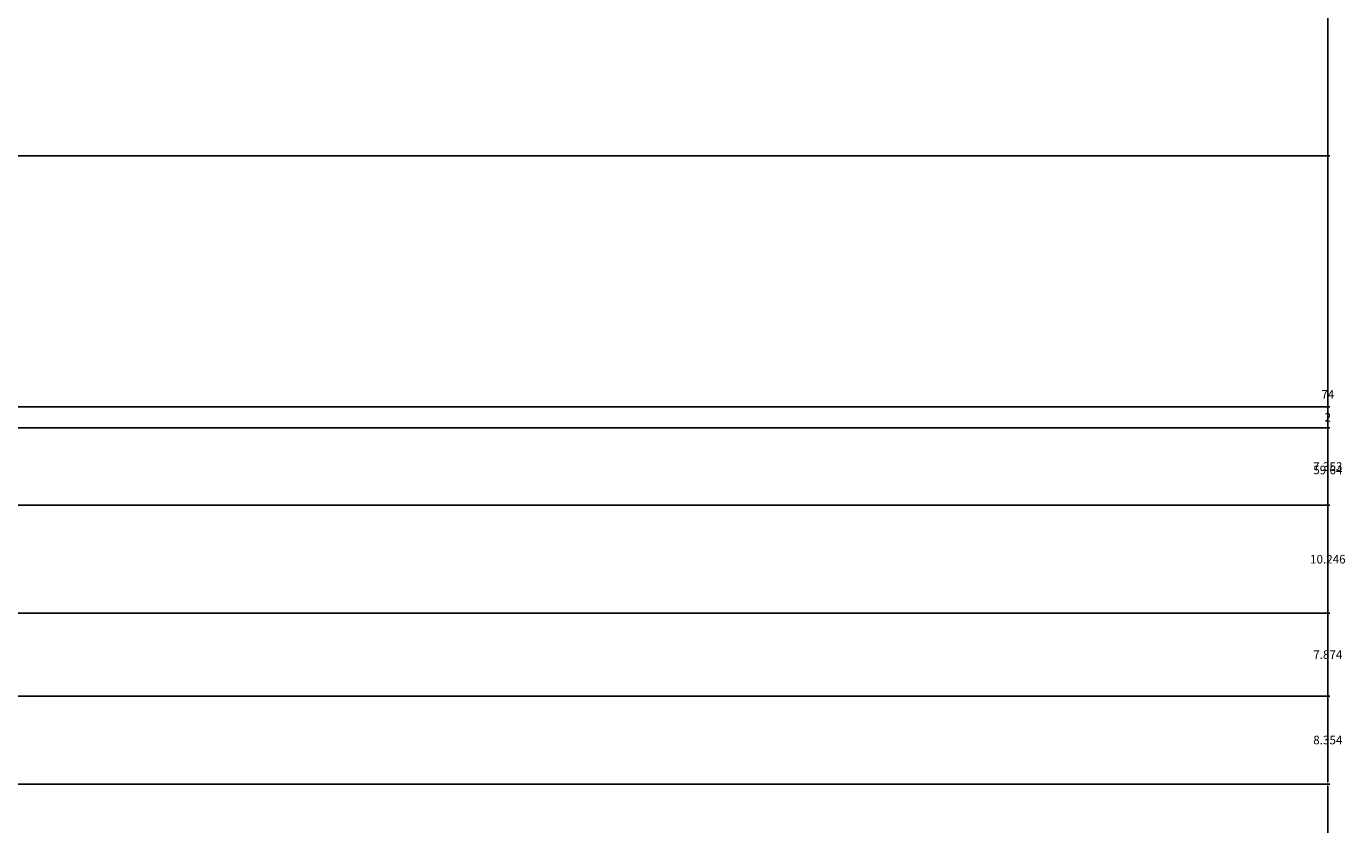
# Model space of a CAD drawing. Units: inches. Extents: x 36 to 594, y 79 to 831.
# Tile 29 of 30: x 469 to 594, y 590 to 666. Entities that reach past the tile are written whole.
import ezdxf

# ---------------------------------------------------------------- set-up
doc = ezdxf.new("R2010")
doc.units = ezdxf.units.IN
doc.header["$MEASUREMENT"] = 0
doc.layers.add('A-ANNO-DIMS', color=2, linetype='Continuous', lineweight=18)
doc.styles.get("Standard").update_dxf_attribs({"font": 'arial.ttf'})
doc.dimstyles.get("Standard").update_dxf_attribs({"dimtxt": 0.8125, "dimasz": 0.18, "dimexe": 0.18, "dimexo": 0.0625, "dimgap": 0.09, "dimtad": 0, "dimtih": 1, "dimtoh": 1, "dimdec": 4, "dimzin": 0, "dimdsep": 46, "dimlunit": 4, "dimtxsty": 'Standard', "dimcen": 0.09, "dimadec": 0, "dimazin": 0, "dimtfac": 1, "dimtdec": 4, "dimtofl": 0, "dimtmove": 0, "dimatfit": 3, "dimfxl": 1, "dimtolj": 1, "dimtzin": 0, "dimarcsym": 0})

# ---------------------------------------------------------------- blocks, each defined once
blk = doc.blocks.new('*D35')
at = {"layer": 'A-ANNO-DIMS', "color": 0, "lineweight": -2, "transparency": 16777216}
for p, q in [((424.56, 594.21), (592.85, 594.21)), ((592.67, 594.03), (592.67, 522.71)), ((592.67, 450.39), (592.67, 521.71)), ((448.45, 450.21), (592.85, 450.21))]:
    blk.add_line(p, q, dxfattribs=at)
at = {"layer": 'A-ANNO-DIMS', "color": 0, "transparency": 16777216}
for points in [[(592.64, 594.03), (592.7, 594.03), (592.67, 594.21)], [(592.64, 450.39), (592.7, 450.39), (592.67, 450.21)]]:
    blk.add_solid(points, dxfattribs=at)
at = {"layer": 'Defpoints', "color": 0, "transparency": 16777216}
for p in [(424.5, 594.21), (592.67, 594.21), (448.39, 450.21)]:
    blk.add_point(p, dxfattribs=at)
at = {"layer": 'A-ANNO-DIMS', "color": 0, "transparency": 16777216, "insert": (592.67, 522.21), "char_height": 0.812, "attachment_point": 5}
blk.add_mtext('\\A1;144', dxfattribs=at)
blk = doc.blocks.new('*D36')
at = {"layer": 'A-ANNO-DIMS', "color": 0, "lineweight": -2, "transparency": 16777216}
for p, q in [((448.452274, 668.212359), (592.848908, 668.212359)), ((592.668908, 668.032359), (592.668908, 631.708609)), ((592.668908, 594.392359), (592.668908, 630.716109)), ((424.55834, 594.212359), (592.848908, 594.212359))]:
    blk.add_line(p, q, dxfattribs=at)
at = {"layer": 'A-ANNO-DIMS', "color": 0, "transparency": 16777216}
for points in [[(592.638908, 668.032359), (592.698908, 668.032359), (592.668908, 668.212359)], [(592.638908, 594.392359), (592.698908, 594.392359), (592.668908, 594.212359)]]:
    blk.add_solid(points, dxfattribs=at)
at = {"layer": 'Defpoints', "color": 0, "transparency": 16777216}
for p in [(448.389774, 668.212359), (592.668908, 668.212359), (424.49584, 594.212359)]:
    blk.add_point(p, dxfattribs=at)
at = {"layer": 'A-ANNO-DIMS', "color": 0, "transparency": 16777216, "insert": (592.668908, 631.212359), "char_height": 0.8125, "attachment_point": 5}
blk.add_mtext('\\A1;74', dxfattribs=at)
blk = doc.blocks.new('*D40')
at = {"layer": 'A-ANNO-DIMS', "color": 0, "lineweight": -2, "transparency": 16777216}
for p, q in [((413.27, 653.86), (592.85, 653.86)), ((592.67, 653.68), (592.67, 624.54)), ((592.67, 594.39), (592.67, 623.53)), ((424.56, 594.21), (592.85, 594.21))]:
    blk.add_line(p, q, dxfattribs=at)
at = {"layer": 'A-ANNO-DIMS', "color": 0, "transparency": 16777216}
for points in [[(592.64, 653.68), (592.7, 653.68), (592.67, 653.86)], [(592.64, 594.39), (592.7, 594.39), (592.67, 594.21)]]:
    blk.add_solid(points, dxfattribs=at)
at = {"layer": 'Defpoints', "color": 0, "transparency": 16777216}
for p in [(413.2, 653.86), (592.67, 653.86), (424.5, 594.21)]:
    blk.add_point(p, dxfattribs=at)
at = {"layer": 'A-ANNO-DIMS', "color": 0, "transparency": 16777216, "insert": (592.67, 624.03), "char_height": 0.812, "attachment_point": 5}
blk.add_mtext('\\A1;59.64', dxfattribs=at)
blk = doc.blocks.new('*D117')
at = {"layer": 'A-ANNO-DIMS', "color": 0, "lineweight": -2, "transparency": 16777216}
for p, q in [((341.9, 602.57), (592.85, 602.57)), ((592.67, 602.39), (592.67, 598.89)), ((592.67, 594.39), (592.67, 597.88)), ((341.9, 594.21), (592.85, 594.21))]:
    blk.add_line(p, q, dxfattribs=at)
at = {"layer": 'A-ANNO-DIMS', "color": 0, "transparency": 16777216}
for points in [[(592.64, 602.39), (592.7, 602.39), (592.67, 602.57)], [(592.64, 594.39), (592.7, 594.39), (592.67, 594.21)]]:
    blk.add_solid(points, dxfattribs=at)
at = {"layer": 'Defpoints', "color": 0, "transparency": 16777216}
for p in [(341.84, 602.57), (592.67, 602.57), (341.84, 594.21)]:
    blk.add_point(p, dxfattribs=at)
at = {"layer": 'A-ANNO-DIMS', "color": 0, "transparency": 16777216, "insert": (592.67, 598.39), "char_height": 0.812, "attachment_point": 5}
blk.add_mtext('\\A1;8.354', dxfattribs=at)
blk = doc.blocks.new('*D118')
at = {"layer": 'A-ANNO-DIMS', "color": 0, "lineweight": -2, "transparency": 16777216}
for p, q in [((341.9, 610.44), (592.85, 610.44)), ((592.67, 610.26), (592.67, 607.01)), ((592.67, 602.75), (592.67, 606)), ((341.9, 602.57), (592.85, 602.57))]:
    blk.add_line(p, q, dxfattribs=at)
at = {"layer": 'A-ANNO-DIMS', "color": 0, "transparency": 16777216}
for points in [[(592.64, 610.26), (592.7, 610.26), (592.67, 610.44)], [(592.64, 602.75), (592.7, 602.75), (592.67, 602.57)]]:
    blk.add_solid(points, dxfattribs=at)
at = {"layer": 'Defpoints', "color": 0, "transparency": 16777216}
for p in [(341.84, 610.44), (592.67, 610.44), (341.84, 602.57)]:
    blk.add_point(p, dxfattribs=at)
at = {"layer": 'A-ANNO-DIMS', "color": 0, "transparency": 16777216, "insert": (592.67, 606.5), "char_height": 0.812, "attachment_point": 5}
blk.add_mtext('\\A1;7.874', dxfattribs=at)
blk = doc.blocks.new('*D119')
at = {"layer": 'A-ANNO-DIMS', "color": 0, "lineweight": -2, "transparency": 16777216}
for p, q in [((341.9, 620.69), (592.85, 620.69)), ((592.67, 620.51), (592.67, 616.07)), ((592.67, 610.62), (592.67, 615.06)), ((341.9, 610.44), (592.85, 610.44))]:
    blk.add_line(p, q, dxfattribs=at)
at = {"layer": 'A-ANNO-DIMS', "color": 0, "transparency": 16777216}
for points in [[(592.64, 620.51), (592.7, 620.51), (592.67, 620.69)], [(592.64, 610.62), (592.7, 610.62), (592.67, 610.44)]]:
    blk.add_solid(points, dxfattribs=at)
at = {"layer": 'Defpoints', "color": 0, "transparency": 16777216}
for p in [(341.84, 620.69), (592.67, 620.69), (341.84, 610.44)]:
    blk.add_point(p, dxfattribs=at)
at = {"layer": 'A-ANNO-DIMS', "color": 0, "transparency": 16777216, "insert": (592.67, 615.56), "char_height": 0.812, "attachment_point": 5}
blk.add_mtext('\\A1;10.246', dxfattribs=at)
blk = doc.blocks.new('*D120')
at = {"layer": 'A-ANNO-DIMS', "color": 0, "lineweight": -2, "transparency": 16777216}
for p, q in [((341.9, 628.04), (592.85, 628.04)), ((592.67, 627.86), (592.67, 624.87)), ((592.67, 620.87), (592.67, 623.86)), ((341.9, 620.69), (592.85, 620.69))]:
    blk.add_line(p, q, dxfattribs=at)
at = {"layer": 'A-ANNO-DIMS', "color": 0, "transparency": 16777216}
for points in [[(592.64, 627.86), (592.7, 627.86), (592.67, 628.04)], [(592.64, 620.87), (592.7, 620.87), (592.67, 620.69)]]:
    blk.add_solid(points, dxfattribs=at)
at = {"layer": 'Defpoints', "color": 0, "transparency": 16777216}
for p in [(341.84, 628.04), (592.67, 628.04), (341.84, 620.69)]:
    blk.add_point(p, dxfattribs=at)
at = {"layer": 'A-ANNO-DIMS', "color": 0, "transparency": 16777216, "insert": (592.67, 624.36), "char_height": 0.812, "attachment_point": 5}
blk.add_mtext('\\A1;7.353', dxfattribs=at)
blk = doc.blocks.new('*D121')
at = {"layer": 'A-ANNO-DIMS', "color": 0, "lineweight": -2, "transparency": 16777216}
for p, q in [((341.9, 630.04), (592.85, 630.04)), ((592.67, 629.86), (592.67, 629.54)), ((341.9, 628.04), (592.85, 628.04)), ((592.67, 628.22), (592.67, 628.54))]:
    blk.add_line(p, q, dxfattribs=at)
at = {"layer": 'A-ANNO-DIMS', "color": 0, "transparency": 16777216}
for points in [[(592.64, 629.86), (592.7, 629.86), (592.67, 630.04)], [(592.64, 628.22), (592.7, 628.22), (592.67, 628.04)]]:
    blk.add_solid(points, dxfattribs=at)
at = {"layer": 'Defpoints', "color": 0, "transparency": 16777216}
for p in [(341.84, 630.04), (592.67, 630.04), (341.84, 628.04)]:
    blk.add_point(p, dxfattribs=at)
at = {"layer": 'A-ANNO-DIMS', "color": 0, "transparency": 16777216, "insert": (592.67, 629.04), "char_height": 0.812, "attachment_point": 5}
blk.add_mtext('\\A1;2', dxfattribs=at)

msp = doc.modelspace()

# ---------------------------------------------------------------- dimensions: what is measured, and where the dimension line sits
at = {"layer": 'A-ANNO-DIMS'}
for base, p1, p2, override, picture, middle in [((592.6689, 668.2124), (424.4958, 594.2124), (448.3898, 668.2124), {"dimdec": 0, "dimlfac": 1, "dimrnd": 0, "dimzin": 0, "dimdsep": 46, "dimlunit": 2}, '*D36', (592.6689, 631.2124)), ((592.6689, 653.8563), (424.4958, 594.2124), (413.2033, 653.8563), {"dimdec": 2, "dimlfac": 1, "dimrnd": 0, "dimzin": 0, "dimdsep": 46, "dimlunit": 2}, '*D40', (592.6689, 624.0344)), ((592.6689, 630.0394), (341.8367, 628.0394), (341.8367, 630.0394), {"dimdec": 0, "dimlfac": 1, "dimrnd": 0, "dimzin": 0, "dimdsep": 46, "dimlunit": 2}, '*D121', (592.6689, 629.0394)), ((592.6689, 628.0394), (341.8367, 620.6866), (341.8367, 628.0394), {"dimdec": 3, "dimlfac": 1, "dimrnd": 0, "dimzin": 0, "dimdsep": 46, "dimlunit": 2}, '*D120', (592.6689, 624.363)), ((592.6689, 620.6866), (341.8367, 610.4402), (341.8367, 620.6866), {"dimdec": 3, "dimlfac": 1, "dimrnd": 0, "dimzin": 0, "dimdsep": 46, "dimlunit": 2}, '*D119', (592.6689, 615.5634)), ((592.66891, 610.44025), (341.83669, 602.56672), (341.83669, 610.44025), {"dimdec": 3, "dimlfac": 1, "dimrnd": 0, "dimzin": 0, "dimdsep": 46, "dimlunit": 2}, '*D118', (592.66891, 606.50348)), ((592.6689, 602.5667), (341.8367, 594.2124), (341.8367, 602.5667), {"dimdec": 3, "dimlfac": 1, "dimrnd": 0, "dimzin": 0, "dimdsep": 46, "dimlunit": 2}, '*D117', (592.6689, 598.3895)), ((592.6689, 594.2124), (448.3898, 450.2124), (424.4958, 594.2124), {"dimdec": 0, "dimlfac": 1, "dimrnd": 0, "dimzin": 0, "dimdsep": 46, "dimlunit": 2}, '*D35', (592.6689, 522.2124))]:
    dim = msp.add_linear_dim(base=base, p1=p1, p2=p2, angle=90, dimstyle='Standard', override=override, dxfattribs=at)
    dim.commit()
    dim.dimension.update_dxf_attribs({"geometry": picture, "text_midpoint": middle})

doc.saveas('drawing.dxf')
